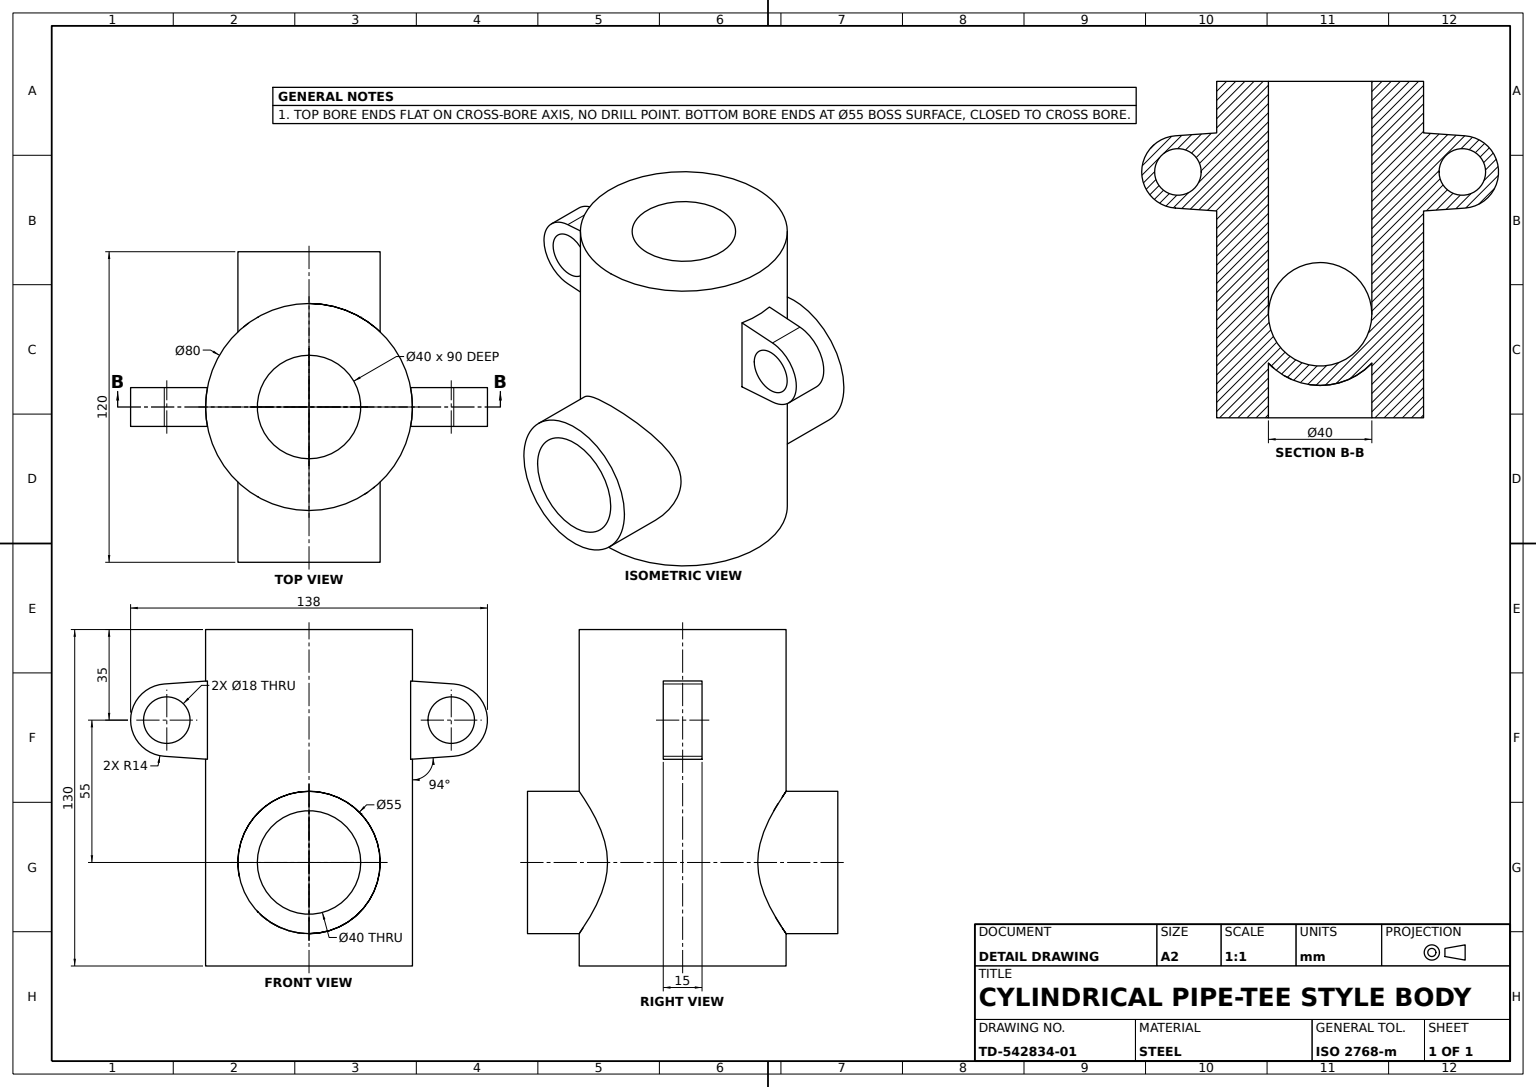
from build123d import *
from build123d.topology import SkipClean

# Parameters (mm, degrees)
MAIN_BODY_SKETCH_R     = 40
MAIN_BODY_SKETCH_R_2   = 20
MAIN_BODY_DEPTH        = 130
CROSS_BOSS_SKETCH_R    = 27.5
CROSS_BOSS_SKETCH_R_2  = 20
CROSS_BOSS_DEPTH       = 60
MOUNTING_LUGS_SKETCH_R = 9
MOUNTING_LUGS_DEPTH    = 7.5
TOP_START              = -90
TOP_BORE_SKETCH_R      = 20
TOP_BORE_DEPTH         = 90
CROSS_START            = -150
CROSS_BORE_SKETCH_R    = 20
CROSS_BORE_DEPTH       = 150


with BuildPart() as part:
    # Main Body Sketch → Main Body (new body)
    with BuildSketch(Plane(origin=(0, 0, 0), x_dir=(1, 0, 0), z_dir=(0, 1, 0))):
        with Locations(Location((0, 0, 0), (0, 0, 270))):
            Circle(MAIN_BODY_SKETCH_R)
        with Locations(Location((0, 0, 0), (0, 0, 270))):
            Circle(MAIN_BODY_SKETCH_R_2, mode=Mode.SUBTRACT)
    extrude(amount=MAIN_BODY_DEPTH)

    # Cross Boss Sketch → Cross Boss (add, symmetric)
    with BuildSketch(Plane.XY):
        with Locations(Location((0, 40, 0), (0, 0, 180))):
            Circle(CROSS_BOSS_SKETCH_R)
        with Locations(Location((0, 40, 0), (0, 0, 180))):
            Circle(CROSS_BOSS_SKETCH_R_2, mode=Mode.SUBTRACT)
    extrude(amount=CROSS_BOSS_DEPTH, both=True)

    # Mounting Lugs Sketch → Mounting Lugs (add, symmetric)
    # profile 1 of 2: a face of its own
    with BuildSketch(Plane.XY):
        with BuildLine():
            Line((-19.924205085, 78.513074912), (0, 78.666038311))
            Line((0, 78.666038311), (0, 111.258543393))
            Line((0, 111.258543393), (-23.164655311, 111.260330734))
            Line((-23.164655311, 111.260330734), (-55.976590632, 108.965896704))
            ThreePointArc((-55.976590632, 108.965896704), (-69, 95), (-55.976590632, 81.034103296))
            Line((-55.976590632, 81.034103296), (-19.924205085, 78.513074912))
        make_face()
        with Locations((-55, 95)):
            Circle(MOUNTING_LUGS_SKETCH_R, mode=Mode.SUBTRACT)
    # profile 2 of 2: a face of its own
    with BuildSketch(Plane.XY):
        with BuildLine():
            Line((0, 111.258543393), (0, 78.666038311))
            Line((0, 78.666038311), (24.838727552, 78.8567318))
            Line((24.838727552, 78.8567318), (55.976590632, 81.034103296))
            ThreePointArc((55.976590632, 81.034103296), (69, 95), (55.976590632, 108.965896704))
            Line((55.976590632, 108.965896704), (23.215832129, 111.256752103))
            Line((23.215832129, 111.256752103), (0, 111.258543393))
        make_face()
        with Locations((55, 95)):
            Circle(MOUNTING_LUGS_SKETCH_R, mode=Mode.SUBTRACT)
    extrude(amount=MOUNTING_LUGS_DEPTH, both=True)

    # Top Bore Sketch → Top Bore (cut)
    with SkipClean():  # the faces are left unmerged after this step: merging them gives an invalid solid
        with BuildSketch(Plane(origin=(0, 130, 0), x_dir=(1, 0, 0), z_dir=(0, 1, 0)).offset(TOP_START)):
            with Locations(Location((0, 0, 0), (0, 0, 180))):
                Circle(TOP_BORE_SKETCH_R)
        extrude(amount=TOP_BORE_DEPTH, mode=Mode.SUBTRACT)

    # Cross Bore Sketch → Cross Bore (cut)
    with SkipClean():  # the faces are left unmerged after this step: merging them gives an invalid solid
        with BuildSketch(Plane.XY.offset(60).offset(CROSS_START)):
            with Locations((0, 40)):
                Circle(CROSS_BORE_SKETCH_R)
        extrude(amount=CROSS_BORE_DEPTH, mode=Mode.SUBTRACT)


solid = part.part
